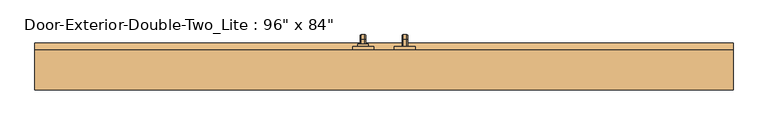
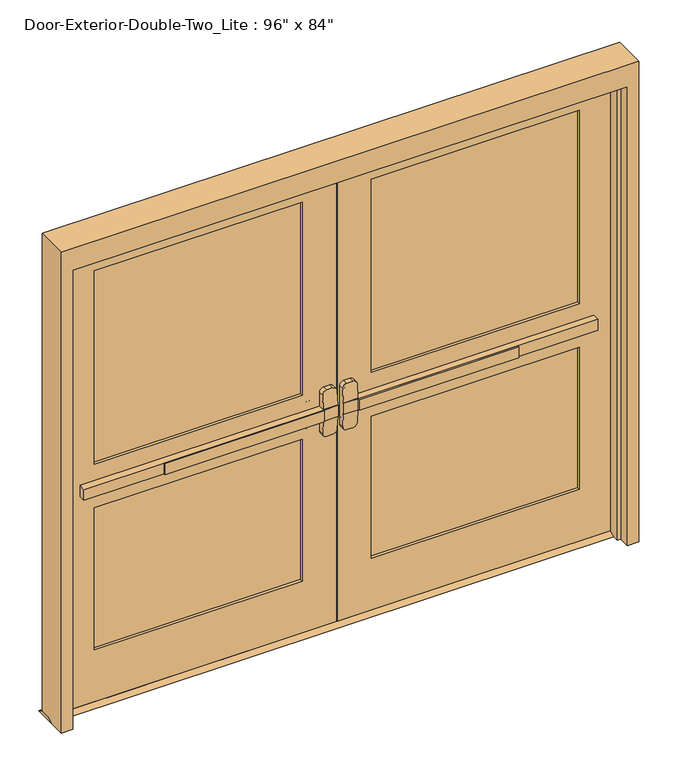
"""IFC4 building model written with IfcOpenShell, lengths in millimetres: door geometry."""

from ifc_helpers import new_model, si_unit, point, frame, frame_2d, origin, place, context, project, spatial, polyline, circle_curve, ellipse_curve, trimmed, segment, composite_curve, outline, extrude, faceted_brep, source, transform, mapped, element, save
from ifc_brep_helpers import plane_surface, cylinder_surface, revolved_surface, advanced_brep


def door_14451ac2(model_context):
    return source(origin(), model_context, "Body", "SolidModel", [
        extrude(outline(polyline([(-778.9333333, 0.0), (-778.9333333, 6.35), (-76.2, 6.35), (-76.2, 0.0), (-778.9333333, 0.0)])), frame((0.0, 0.0, 990.6), z_axis=(0.0, 0.0, 1.0), x_axis=(1.0, 0.0, 0.0)), (0.0, 0.0, 1.0), 50.8),
        advanced_brep(
        [(-12.7, 6.35, 1041.4), (-76.2, 6.35, 1041.4), (-1130.3, 6.35, 1041.4), (-1130.3, 6.35, 990.6), (-76.2, 6.35, 990.6), (-12.7, 6.35, 990.6), (-1130.3, 38.1, 1041.4), (-76.2, 38.1, 1041.4), (-76.2, 38.1, 1104.9), (-57.15, 38.1, 1123.95), (-31.75, 38.1, 1123.95), (-12.7, 38.1, 1104.9), (-12.7, 38.1, 927.1), (-31.75, 38.1, 908.05), (-57.15, 38.1, 908.05), (-76.2, 38.1, 927.1), (-76.2, 38.1, 990.6), (-1130.3, 38.1, 990.6), (-12.7, 9.5252467, 1041.4), (-76.2, 9.5252467, 1041.4), (-12.7, 9.5252467, 990.6), (-12.7, 14.5354269, 927.1), (-12.7, 14.5354269, 1104.9), (-76.2, 9.5252467, 990.6), (-76.2, 14.5354269, 1104.9), (-76.2, 14.5354269, 927.1), (-57.15, 16.038481, 1123.95), (-31.75, 16.038481, 1123.95), (-31.75, 16.038481, 908.05), (-57.15, 16.038481, 908.05)],
        [
            (0, 1),
            (1, 2),
            (2, 3),
            (3, 4),
            (4, 5),
            (5, 0),
            (6, 7),
            (7, 8),
            (8, 9, circle_curve(frame((-57.15, 38.1, 1104.9), z_axis=(0.0, 1.0, 0.0), x_axis=(-1.0, 0.0, 0.0)), 19.05)),
            (9, 10),
            (10, 11, circle_curve(frame((-31.75, 38.1, 1104.9), z_axis=(0.0, 1.0, 0.0), x_axis=(-1.0, 0.0, 0.0)), 19.05)),
            (11, 12),
            (12, 13, circle_curve(frame((-31.75, 38.1, 927.1), z_axis=(0.0, 1.0, 0.0), x_axis=(-1.0, 0.0, 0.0)), 19.05)),
            (13, 14),
            (14, 15, circle_curve(frame((-57.15, 38.1, 927.1), z_axis=(0.0, 1.0, 0.0), x_axis=(-1.0, 0.0, 0.0)), 19.05)),
            (15, 16),
            (16, 17),
            (17, 6),
            (0, 18),
            (18, 19),
            (19, 7),
            (6, 2),
            (5, 20),
            (20, 21),
            (21, 12),
            (11, 22),
            (22, 18),
            (16, 23),
            (23, 20),
            (3, 17),
            (19, 24),
            (24, 8),
            (15, 25),
            (25, 23),
            (9, 26),
            (26, 27),
            (27, 10),
            (13, 28),
            (28, 29),
            (29, 14),
            (29, 25, ellipse_curve(frame((-57.15, 14.5354269, 927.1), z_axis=(0.0, 0.9969018152893365, 0.07865602756830282), x_axis=(0.0, -0.07865602756830208, 0.9969018152893365)), 19.1092038, 19.05)),
            (24, 26, ellipse_curve(frame((-57.15, 14.5354269, 1104.9), z_axis=(0.0, 0.9969018152893376, -0.07865602756828934), x_axis=(0.0, -0.078656027568288, -0.9969018152893377)), 19.1092038, 19.05)),
            (27, 22, ellipse_curve(frame((-31.75, 14.5354269, 1104.9), z_axis=(0.0, 0.9969018152893376, -0.07865602756828934), x_axis=(0.0, -0.078656027568288, -0.9969018152893377)), 19.1092038, 19.05)),
            (21, 28, ellipse_curve(frame((-31.75, 14.5354269, 927.1), z_axis=(0.0, 0.9969018152893365, 0.07865602756830282), x_axis=(0.0, -0.07865602756830208, 0.9969018152893365)), 19.1092038, 19.05)),
        ],
        [
            plane_surface(frame((-12.7, 6.35, 1041.4), z_axis=(0.0, -1.0, 0.0), x_axis=(1.0, 0.0, 0.0))),
            plane_surface(frame((-12.7, 38.1, 1041.4), z_axis=(0.0, 1.0, 0.0), x_axis=(-1.0, 0.0, 0.0))),
            plane_surface(frame((-1130.3, 6.35, 1041.4), z_axis=(0.0, 0.0, 1.0), x_axis=(0.0, 1.0, 0.0))),
            plane_surface(frame((-12.7, 6.35, 1041.4), z_axis=(1.0, 0.0, 0.0), x_axis=(0.0, 1.0, 0.0))),
            plane_surface(frame((-12.7, 6.35, 990.6), z_axis=(0.0, 0.0, -1.0), x_axis=(0.0, 1.0, 0.0))),
            plane_surface(frame((-1130.3, 6.35, 990.6), z_axis=(-1.0, 0.0, 0.0), x_axis=(0.0, 1.0, 0.0))),
            plane_surface(frame((-76.2, 9.5252467, 927.1), z_axis=(-1.0, 0.0, 0.0), x_axis=(0.0, 1.0, 0.0))),
            plane_surface(frame((-57.15, 9.5252467, 1123.95), z_axis=(0.0, 0.0, 1.0), x_axis=(0.0, 1.0, 0.0))),
            plane_surface(frame((-31.75, 9.5252467, 908.05), z_axis=(0.0, 0.0, -1.0), x_axis=(0.0, 1.0, 0.0))),
            cylinder_surface(frame((-57.15, 38.1, 927.1), z_axis=(0.0, -1.0, 0.0), x_axis=(-1.0, 0.0, 0.0)), 19.05),
            cylinder_surface(frame((-57.15, 38.1, 1104.9), z_axis=(0.0, -1.0, 0.0), x_axis=(-1.0, 0.0, 0.0)), 19.05),
            cylinder_surface(frame((-31.75, 38.1, 1104.9), z_axis=(0.0, -1.0, 0.0), x_axis=(-1.0, 0.0, 0.0)), 19.05),
            cylinder_surface(frame((-31.75, 38.1, 927.1), z_axis=(0.0, -1.0, 0.0), x_axis=(-1.0, 0.0, 0.0)), 19.05),
            plane_surface(frame((-76.2, 9.5252467, 1041.4), z_axis=(0.0, -0.9969018152893376, 0.07865602756828934), x_axis=(1.0, 0.0, 0.0))),
            plane_surface(frame((-76.2, 16.038481, 908.05), z_axis=(0.0, -0.9969018152893365, -0.07865602756830282), x_axis=(1.0, 0.0, 0.0))),
        ],
        [
            (0, [[1, 2, 3, 4, 5, 6]]),
            (1, [[7, 8, 9, 10, 11, 12, 13, 14, 15, 16, 17, 18]]),
            (2, [[-2, -1, 19, 20, 21, -7, 22]]),
            (3, [[23, 24, 25, -12, 26, 27, -19, -6]]),
            (4, [[-17, 28, 29, -23, -5, -4, 30]]),
            (5, [[-22, -18, -30, -3]]),
            (6, [[-21, 31, 32, -8]]),
            (6, [[33, 34, -28, -16]]),
            (7, [[35, 36, 37, -10]]),
            (8, [[38, 39, 40, -14]]),
            (9, [[-40, 41, -33, -15]]),
            (10, [[-32, 42, -35, -9]]),
            (11, [[-37, 43, -26, -11]]),
            (12, [[-25, 44, -38, -13]]),
            (13, [[-27, -43, -36, -42, -31, -20]]),
            (14, [[-29, -34, -41, -39, -44, -24]]),
        ],
    ),
        extrude(outline(polyline([(82.55, 12.7), (107.95, 0.0), (12.7, 0.0), (38.1, 12.7), (82.55, 12.7)])), frame((-1270.0, 0.0, 0.0), z_axis=(1.0, 0.0, 0.0), x_axis=(0.0, 1.0, 0.0)), (0.0, 0.0, 1.0), 2540.0),
        extrude(outline(polyline([(778.9333333, 0.0), (76.2, 0.0), (76.2, 6.35), (778.9333333, 6.35), (778.9333333, 0.0)])), frame((0.0, 0.0, 990.6), z_axis=(0.0, 0.0, 1.0), x_axis=(1.0, 0.0, 0.0)), (0.0, 0.0, 1.0), 50.8),
        advanced_brep(
        [(12.7, 6.35, 1041.4), (12.7, 6.35, 990.6), (76.2, 6.35, 990.6), (1130.3, 6.35, 990.6), (1130.3, 6.35, 1041.4), (76.2, 6.35, 1041.4), (1130.3, 38.1, 1041.4), (1130.3, 38.1, 990.6), (76.2, 38.1, 990.6), (76.2, 38.1, 927.1), (57.15, 38.1, 908.05), (31.75, 38.1, 908.05), (12.7, 38.1, 927.1), (12.7, 38.1, 1104.9), (31.75, 38.1, 1123.95), (57.15, 38.1, 1123.95), (76.2, 38.1, 1104.9), (76.2, 38.1, 1041.4), (76.2, 9.5252467, 1041.4), (12.7, 9.5252467, 1041.4), (12.7, 14.5354269, 1104.9), (12.7, 14.5354269, 927.1), (12.7, 9.5252467, 990.6), (76.2, 9.5252467, 990.6), (76.2, 14.5354269, 927.1), (76.2, 14.5354269, 1104.9), (31.75, 16.038481, 1123.95), (57.15, 16.038481, 1123.95), (57.15, 16.038481, 908.05), (31.75, 16.038481, 908.05)],
        [
            (0, 1),
            (1, 2),
            (2, 3),
            (3, 4),
            (4, 5),
            (5, 0),
            (6, 7),
            (7, 8),
            (8, 9),
            (9, 10, circle_curve(frame((57.15, 38.1, 927.1), z_axis=(0.0, 1.0, 0.0), x_axis=(1.0, 0.0, 0.0)), 19.05)),
            (10, 11),
            (11, 12, circle_curve(frame((31.75, 38.1, 927.1), z_axis=(0.0, 1.0, 0.0), x_axis=(1.0, 0.0, 0.0)), 19.05)),
            (12, 13),
            (13, 14, circle_curve(frame((31.75, 38.1, 1104.9), z_axis=(0.0, 1.0, 0.0), x_axis=(1.0, 0.0, 0.0)), 19.05)),
            (14, 15),
            (15, 16, circle_curve(frame((57.15, 38.1, 1104.9), z_axis=(0.0, 1.0, 0.0), x_axis=(1.0, 0.0, 0.0)), 19.05)),
            (16, 17),
            (17, 6),
            (4, 6),
            (17, 18),
            (18, 19),
            (19, 0),
            (19, 20),
            (20, 13),
            (12, 21),
            (21, 22),
            (22, 1),
            (7, 3),
            (22, 23),
            (23, 8),
            (23, 24),
            (24, 9),
            (16, 25),
            (25, 18),
            (14, 26),
            (26, 27),
            (27, 15),
            (10, 28),
            (28, 29),
            (29, 11),
            (24, 28, ellipse_curve(frame((57.15, 14.5354269, 927.1), z_axis=(0.0, 0.9969018152893365, 0.07865602756830282), x_axis=(0.0, -0.07865602756830208, 0.9969018152893365)), 19.1092038, 19.05)),
            (27, 25, ellipse_curve(frame((57.15, 14.5354269, 1104.9), z_axis=(0.0, 0.9969018152893376, -0.07865602756828934), x_axis=(0.0, -0.078656027568288, -0.9969018152893377)), 19.1092038, 19.05)),
            (20, 26, ellipse_curve(frame((31.75, 14.5354269, 1104.9), z_axis=(0.0, 0.9969018152893376, -0.07865602756828934), x_axis=(0.0, -0.078656027568288, -0.9969018152893377)), 19.1092038, 19.05)),
            (29, 21, ellipse_curve(frame((31.75, 14.5354269, 927.1), z_axis=(0.0, 0.9969018152893365, 0.07865602756830282), x_axis=(0.0, -0.07865602756830208, 0.9969018152893365)), 19.1092038, 19.05)),
        ],
        [
            plane_surface(frame((12.7, 6.35, 1041.4), z_axis=(0.0, -1.0, 0.0), x_axis=(-1.0, 0.0, 0.0))),
            plane_surface(frame((12.7, 38.1, 1041.4), z_axis=(0.0, 1.0, 0.0), x_axis=(1.0, 0.0, 0.0))),
            plane_surface(frame((1130.3, 6.35, 1041.4), z_axis=(0.0, 0.0, 1.0), x_axis=(0.0, 1.0, 0.0))),
            plane_surface(frame((12.7, 6.35, 1041.4), z_axis=(-1.0, 0.0, 0.0), x_axis=(0.0, 1.0, 0.0))),
            plane_surface(frame((12.7, 6.35, 990.6), z_axis=(0.0, 0.0, -1.0), x_axis=(0.0, 1.0, 0.0))),
            plane_surface(frame((1130.3, 6.35, 990.6), z_axis=(1.0, 0.0, 0.0), x_axis=(0.0, 1.0, 0.0))),
            plane_surface(frame((76.2, 9.5252467, 927.1), z_axis=(1.0, 0.0, 0.0), x_axis=(0.0, 1.0, 0.0))),
            plane_surface(frame((57.15, 9.5252467, 1123.95), z_axis=(0.0, 0.0, 1.0), x_axis=(0.0, 1.0, 0.0))),
            plane_surface(frame((31.75, 9.5252467, 908.05), z_axis=(0.0, 0.0, -1.0), x_axis=(0.0, 1.0, 0.0))),
            cylinder_surface(frame((57.15, 38.1, 927.1), z_axis=(0.0, -1.0, 0.0), x_axis=(1.0, 0.0, 0.0)), 19.05),
            cylinder_surface(frame((57.15, 38.1, 1104.9), z_axis=(0.0, -1.0, 0.0), x_axis=(1.0, 0.0, 0.0)), 19.05),
            cylinder_surface(frame((31.75, 38.1, 1104.9), z_axis=(0.0, -1.0, 0.0), x_axis=(1.0, 0.0, 0.0)), 19.05),
            cylinder_surface(frame((31.75, 38.1, 927.1), z_axis=(0.0, -1.0, 0.0), x_axis=(1.0, 0.0, 0.0)), 19.05),
            plane_surface(frame((76.2, 9.5252467, 1041.4), z_axis=(0.0, -0.9969018152893376, 0.07865602756828934), x_axis=(-1.0, 0.0, 0.0))),
            plane_surface(frame((76.2, 16.038481, 908.05), z_axis=(0.0, -0.9969018152893365, -0.07865602756830282), x_axis=(-1.0, 0.0, 0.0))),
        ],
        [
            (0, [[1, 2, 3, 4, 5, 6]]),
            (1, [[7, 8, 9, 10, 11, 12, 13, 14, 15, 16, 17, 18]]),
            (2, [[19, -18, 20, 21, 22, -6, -5]]),
            (3, [[-1, -22, 23, 24, -13, 25, 26, 27]]),
            (4, [[28, -3, -2, -27, 29, 30, -8]]),
            (5, [[-4, -28, -7, -19]]),
            (6, [[-9, -30, 31, 32]]),
            (6, [[-17, 33, 34, -20]]),
            (7, [[-15, 35, 36, 37]]),
            (8, [[-11, 38, 39, 40]]),
            (9, [[-10, -32, 41, -38]]),
            (10, [[-16, -37, 42, -33]]),
            (11, [[-14, -24, 43, -35]]),
            (12, [[-12, -40, 44, -25]]),
            (13, [[-21, -34, -42, -36, -43, -23]]),
            (14, [[-26, -44, -39, -41, -31, -29]]),
        ],
    ),
        advanced_brep(
        [(66.2, 95.25, 1017.190625), (66.2, 95.25, 1014.809375), (69.771875, 95.25, 1011.2375), (82.6284594, 95.25, 1011.2375), (86.2, 95.25, 1014.8090406), (86.2, 95.25, 1017.190625), (82.628125, 95.25, 1020.7625), (69.771875, 95.25, 1020.7625), (66.2, 95.25, 887.809375), (69.771875, 95.25, 884.2375), (82.628125, 95.25, 884.2375), (86.2, 95.25, 887.809375), (86.2, 95.25, 890.1909594), (82.6284594, 95.25, 893.7625), (69.771875, 95.25, 893.7625), (66.2, 95.25, 890.190625), (66.2, 120.65, 1017.190625), (66.2, 134.540625, 1003.3), (66.2, 134.540625, 901.7), (66.2, 120.65, 887.809375), (66.2, 120.65, 890.190625), (66.2, 132.159375, 901.7), (66.2, 132.159375, 1003.3), (66.2, 120.65, 1014.809375), (69.771875, 120.65, 1011.2375), (82.6284594, 120.65, 1011.2375), (86.2, 120.65, 1014.8090406), (86.2, 132.1590406, 1003.3), (86.2, 132.1590406, 901.7), (86.2, 120.65, 890.1909594), (86.2, 120.65, 887.809375), (86.2, 134.540625, 901.7), (86.2, 134.540625, 1003.3), (86.2, 120.65, 1017.190625), (82.628125, 120.65, 1020.7625), (69.771875, 120.65, 1020.7625), (69.771875, 128.5875, 1003.3), (82.6284594, 128.5875, 1003.3), (82.628125, 138.1125, 1003.3), (69.771875, 138.1125, 1003.3), (69.771875, 128.5875, 901.7), (82.6284594, 128.5875, 901.7), (82.628125, 138.1125, 901.7), (69.771875, 138.1125, 901.7), (69.771875, 120.65, 893.7625), (82.6284594, 120.65, 893.7625), (82.628125, 120.65, 884.2375), (69.771875, 120.65, 884.2375)],
        [
            (0, 1),
            (1, 2, circle_curve(frame((69.771875, 95.25, 1014.809375), z_axis=(0.0, -1.0, 0.0), x_axis=(0.0, 0.0, 1.0)), 3.571875)),
            (2, 3),
            (3, 4, circle_curve(frame((82.6284594, 95.25, 1014.8090406), z_axis=(0.0, -1.0, 0.0), x_axis=(0.0, 0.0, 1.0)), 3.5715406)),
            (4, 5),
            (5, 6, circle_curve(frame((82.628125, 95.25, 1017.190625), z_axis=(0.0, -1.0, 0.0), x_axis=(0.0, 0.0, 1.0)), 3.571875)),
            (6, 7),
            (7, 0, circle_curve(frame((69.771875, 95.25, 1017.190625), z_axis=(0.0, -1.0, 0.0), x_axis=(0.0, 0.0, 1.0)), 3.571875)),
            (8, 9, circle_curve(frame((69.771875, 95.25, 887.809375), z_axis=(0.0, -1.0, 0.0), x_axis=(0.0, 0.0, -1.0)), 3.571875)),
            (9, 10),
            (10, 11, circle_curve(frame((82.628125, 95.25, 887.809375), z_axis=(0.0, -1.0, 0.0), x_axis=(0.0, 0.0, -1.0)), 3.571875)),
            (11, 12),
            (12, 13, circle_curve(frame((82.6284594, 95.25, 890.1909594), z_axis=(0.0, -1.0, 0.0), x_axis=(0.0, 0.0, -1.0)), 3.5715406)),
            (13, 14),
            (14, 15, circle_curve(frame((69.771875, 95.25, 890.190625), z_axis=(0.0, -1.0, 0.0), x_axis=(0.0, 0.0, -1.0)), 3.571875)),
            (15, 8),
            (0, 16),
            (16, 17, circle_curve(frame((66.2, 120.65, 1003.3), z_axis=(-1.0, 0.0, 0.0), x_axis=(0.0, 0.0, 1.0)), 13.890625)),
            (17, 18),
            (18, 19, circle_curve(frame((66.2, 120.65, 901.7), z_axis=(-1.0, 0.0, 0.0), x_axis=(0.0, 1.0, 0.0)), 13.890625)),
            (19, 8),
            (15, 20),
            (20, 21, circle_curve(frame((66.2, 120.65, 901.7), z_axis=(1.0, 0.0, 0.0), x_axis=(0.0, 1.0, 0.0)), 11.509375)),
            (21, 22),
            (22, 23, circle_curve(frame((66.2, 120.65, 1003.3), z_axis=(1.0, 0.0, 0.0), x_axis=(0.0, 0.0, 1.0)), 11.509375)),
            (23, 1),
            (23, 24, circle_curve(frame((69.771875, 120.65, 1014.809375), z_axis=(0.0, -1.0, 0.0), x_axis=(0.0, 0.0, 1.0)), 3.571875)),
            (24, 2),
            (24, 25),
            (25, 3),
            (25, 26, circle_curve(frame((82.6284594, 120.65, 1014.8090406), z_axis=(0.0, -1.0, 0.0), x_axis=(0.0, 0.0, 1.0)), 3.5715406)),
            (26, 4),
            (26, 27, circle_curve(frame((86.2, 120.65, 1003.3), z_axis=(-1.0, 0.0, 0.0), x_axis=(0.0, 0.0, 1.0)), 11.5090406)),
            (27, 28),
            (28, 29, circle_curve(frame((86.2, 120.65, 901.7), z_axis=(-1.0, 0.0, 0.0), x_axis=(0.0, 1.0, 0.0)), 11.5090406)),
            (29, 12),
            (11, 30),
            (30, 31, circle_curve(frame((86.2, 120.65, 901.7), z_axis=(1.0, 0.0, 0.0), x_axis=(0.0, 1.0, 0.0)), 13.890625)),
            (31, 32),
            (32, 33, circle_curve(frame((86.2, 120.65, 1003.3), z_axis=(1.0, 0.0, 0.0), x_axis=(0.0, 0.0, 1.0)), 13.890625)),
            (33, 5),
            (33, 34, circle_curve(frame((82.628125, 120.65, 1017.190625), z_axis=(0.0, -1.0, 0.0), x_axis=(0.0, 0.0, 1.0)), 3.571875)),
            (34, 6),
            (34, 35),
            (35, 7),
            (35, 16, circle_curve(frame((69.771875, 120.65, 1017.190625), z_axis=(0.0, -1.0, 0.0), x_axis=(0.0, 0.0, 1.0)), 3.571875)),
            (36, 24, circle_curve(frame((69.771875, 120.65, 1003.3), z_axis=(1.0, 0.0, 0.0), x_axis=(0.0, 0.0, 1.0)), 7.9375)),
            (22, 36, circle_curve(frame((69.771875, 132.159375, 1003.3), z_axis=(0.0, 0.0, 1.0), x_axis=(0.0, 1.0, 0.0)), 3.571875)),
            (37, 25, circle_curve(frame((82.6284594, 120.65, 1003.3), z_axis=(1.0, 0.0, 0.0), x_axis=(0.0, 0.0, 1.0)), 7.9375)),
            (36, 37),
            (37, 27, circle_curve(frame((82.6284594, 132.1590406, 1003.3), z_axis=(0.0, 0.0, 1.0), x_axis=(0.0, 1.0, 0.0)), 3.5715406)),
            (38, 34, circle_curve(frame((82.628125, 120.65, 1003.3), z_axis=(1.0, 0.0, 0.0), x_axis=(0.0, 0.0, 1.0)), 17.4625)),
            (32, 38, circle_curve(frame((82.628125, 134.540625, 1003.3), z_axis=(0.0, 0.0, 1.0), x_axis=(0.0, 1.0, 0.0)), 3.571875)),
            (39, 35, circle_curve(frame((69.771875, 120.65, 1003.3), z_axis=(1.0, 0.0, 0.0), x_axis=(0.0, 0.0, 1.0)), 17.4625)),
            (38, 39),
            (39, 17, circle_curve(frame((69.771875, 134.540625, 1003.3), z_axis=(0.0, 0.0, 1.0), x_axis=(0.0, 1.0, 0.0)), 3.571875)),
            (21, 40, circle_curve(frame((69.771875, 132.159375, 901.7), z_axis=(0.0, 0.0, 1.0), x_axis=(0.0, 1.0, 0.0)), 3.571875)),
            (40, 36),
            (40, 41),
            (41, 37),
            (41, 28, circle_curve(frame((82.6284594, 132.1590406, 901.7), z_axis=(0.0, 0.0, 1.0), x_axis=(0.0, 1.0, 0.0)), 3.5715406)),
            (31, 42, circle_curve(frame((82.628125, 134.540625, 901.7), z_axis=(0.0, 0.0, 1.0), x_axis=(0.0, 1.0, 0.0)), 3.571875)),
            (42, 38),
            (42, 43),
            (43, 39),
            (43, 18, circle_curve(frame((69.771875, 134.540625, 901.7), z_axis=(0.0, 0.0, 1.0), x_axis=(0.0, 1.0, 0.0)), 3.571875)),
            (44, 40, circle_curve(frame((69.771875, 120.65, 901.7), z_axis=(1.0, 0.0, 0.0), x_axis=(0.0, 1.0, 0.0)), 7.9375)),
            (20, 44, circle_curve(frame((69.771875, 120.65, 890.190625), z_axis=(0.0, 1.0, 0.0), x_axis=(0.0, 0.0, -1.0)), 3.571875)),
            (45, 41, circle_curve(frame((82.6284594, 120.65, 901.7), z_axis=(1.0, 0.0, 0.0), x_axis=(0.0, 1.0, 0.0)), 7.9375)),
            (44, 45),
            (45, 29, circle_curve(frame((82.6284594, 120.65, 890.1909594), z_axis=(0.0, 1.0, 0.0), x_axis=(0.0, 0.0, -1.0)), 3.5715406)),
            (46, 42, circle_curve(frame((82.628125, 120.65, 901.7), z_axis=(1.0, 0.0, 0.0), x_axis=(0.0, 1.0, 0.0)), 17.4625)),
            (30, 46, circle_curve(frame((82.628125, 120.65, 887.809375), z_axis=(0.0, 1.0, 0.0), x_axis=(0.0, 0.0, -1.0)), 3.571875)),
            (47, 43, circle_curve(frame((69.771875, 120.65, 901.7), z_axis=(1.0, 0.0, 0.0), x_axis=(0.0, 1.0, 0.0)), 17.4625)),
            (46, 47),
            (47, 19, circle_curve(frame((69.771875, 120.65, 887.809375), z_axis=(0.0, 1.0, 0.0), x_axis=(0.0, 0.0, -1.0)), 3.571875)),
            (14, 44),
            (13, 45),
            (10, 46),
            (9, 47),
        ],
        [
            plane_surface(frame((76.2, 95.25, 1016.0), z_axis=(0.0, -1.0, 0.0), x_axis=(1.0, 0.0, 0.0))),
            plane_surface(frame((76.2, 95.25, 889.0), z_axis=(0.0, -1.0, 0.0), x_axis=(1.0, 0.0, 0.0))),
            plane_surface(frame((66.2, 95.25, 1017.190625), z_axis=(-1.0, 0.0, 0.0), x_axis=(0.0, 1.0, 0.0))),
            cylinder_surface(frame((69.771875, 95.25, 1014.809375), z_axis=(0.0, -1.0, 0.0), x_axis=(0.0, 0.0, 1.0)), 3.571875),
            plane_surface(frame((69.771875, 95.25, 1011.2375), z_axis=(0.0, 0.0, -1.0), x_axis=(0.0, 1.0, 0.0))),
            cylinder_surface(frame((82.6284594, 95.25, 1014.8090406), z_axis=(0.0, -1.0, 0.0), x_axis=(0.0, 0.0, 1.0)), 3.5715406),
            plane_surface(frame((86.2, 95.25, 1014.8090406), z_axis=(1.0, 0.0, 0.0), x_axis=(0.0, 1.0, 0.0))),
            cylinder_surface(frame((82.628125, 95.25, 1017.190625), z_axis=(0.0, -1.0, 0.0), x_axis=(0.0, 0.0, 1.0)), 3.571875),
            plane_surface(frame((82.628125, 95.25, 1020.7625), z_axis=(0.0, 0.0, 1.0), x_axis=(0.0, 1.0, 0.0))),
            cylinder_surface(frame((69.771875, 95.25, 1017.190625), z_axis=(0.0, -1.0, 0.0), x_axis=(0.0, 0.0, 1.0)), 3.571875),
            revolved_surface(trimmed(ellipse_curve(frame((69.771875, 120.65, 1014.809375), z_axis=(0.0, -1.0, 0.0), x_axis=(0.0, 0.0, 1.0)), 3.571875, 3.571875), [point((66.2, 120.65, 1014.809375))], [point((69.771875, 120.65, 1011.2375))], True, "CARTESIAN"), (76.2, 120.65, 1003.3), (-1.0, 0.0, 0.0)),
            revolved_surface(polyline([(69.771875, 120.65, 1011.2375), (82.6284594, 120.65, 1011.2375)]), (76.2, 120.65, 1003.3), (-1.0, 0.0, 0.0)),
            revolved_surface(trimmed(ellipse_curve(frame((82.6284594, 120.65, 1014.8090406), z_axis=(0.0, -1.0, 0.0), x_axis=(0.0, 0.0, 1.0)), 3.5715406, 3.5715406), [point((82.6284594, 120.65, 1011.2375))], [point((86.2, 120.65, 1014.8090406))], True, "CARTESIAN"), (76.2, 120.65, 1003.3), (-1.0, 0.0, 0.0)),
            revolved_surface(trimmed(ellipse_curve(frame((82.628125, 120.65, 1017.190625), z_axis=(0.0, -1.0, 0.0), x_axis=(0.0, 0.0, 1.0)), 3.571875, 3.571875), [point((86.2, 120.65, 1017.190625))], [point((82.628125, 120.65, 1020.7625))], True, "CARTESIAN"), (76.2, 120.65, 1003.3), (-1.0, 0.0, 0.0)),
            cylinder_surface(frame((76.2, 120.65, 1003.3), z_axis=(-1.0, 0.0, 0.0), x_axis=(0.0, 0.0, 1.0)), 17.4625),
            revolved_surface(trimmed(ellipse_curve(frame((69.771875, 120.65, 1017.190625), z_axis=(0.0, -1.0, 0.0), x_axis=(0.0, 0.0, 1.0)), 3.571875, 3.571875), [point((69.771875, 120.65, 1020.7625))], [point((66.2, 120.65, 1017.190625))], True, "CARTESIAN"), (76.2, 120.65, 1003.3), (-1.0, 0.0, 0.0)),
            cylinder_surface(frame((69.771875, 132.159375, 1003.3), z_axis=(0.0, 0.0, 1.0), x_axis=(0.0, 1.0, 0.0)), 3.571875),
            plane_surface(frame((69.771875, 128.5875, 1003.3), z_axis=(0.0, -1.0, 0.0), x_axis=(0.0, 0.0, -1.0))),
            cylinder_surface(frame((82.6284594, 132.1590406, 1003.3), z_axis=(0.0, 0.0, 1.0), x_axis=(0.0, 1.0, 0.0)), 3.5715406),
            cylinder_surface(frame((82.628125, 134.540625, 1003.3), z_axis=(0.0, 0.0, 1.0), x_axis=(0.0, 1.0, 0.0)), 3.571875),
            plane_surface(frame((82.628125, 138.1125, 1003.3), z_axis=(0.0, 1.0, 0.0), x_axis=(0.0, 0.0, -1.0))),
            cylinder_surface(frame((69.771875, 134.540625, 1003.3), z_axis=(0.0, 0.0, 1.0), x_axis=(0.0, 1.0, 0.0)), 3.571875),
            revolved_surface(trimmed(ellipse_curve(frame((69.771875, 132.159375, 901.7), z_axis=(0.0, 0.0, 1.0), x_axis=(0.0, 1.0, 0.0)), 3.571875, 3.571875), [point((66.2, 132.159375, 901.7))], [point((69.771875, 128.5875, 901.7))], True, "CARTESIAN"), (76.2, 120.65, 901.7), (-1.0, 0.0, 0.0)),
            revolved_surface(polyline([(69.771875, 128.5875, 901.7), (82.6284594, 128.5875, 901.7)]), (76.2, 120.65, 901.7), (-1.0, 0.0, 0.0)),
            revolved_surface(trimmed(ellipse_curve(frame((82.6284594, 132.1590406, 901.7), z_axis=(0.0, 0.0, 1.0), x_axis=(0.0, 1.0, 0.0)), 3.5715406, 3.5715406), [point((82.6284594, 128.5875, 901.7))], [point((86.2, 132.1590406, 901.7))], True, "CARTESIAN"), (76.2, 120.65, 901.7), (-1.0, 0.0, 0.0)),
            revolved_surface(trimmed(ellipse_curve(frame((82.628125, 134.540625, 901.7), z_axis=(0.0, 0.0, 1.0), x_axis=(0.0, 1.0, 0.0)), 3.571875, 3.571875), [point((86.2, 134.540625, 901.7))], [point((82.628125, 138.1125, 901.7))], True, "CARTESIAN"), (76.2, 120.65, 901.7), (-1.0, 0.0, 0.0)),
            cylinder_surface(frame((76.2, 120.65, 901.7), z_axis=(-1.0, 0.0, 0.0), x_axis=(0.0, 1.0, 0.0)), 17.4625),
            revolved_surface(trimmed(ellipse_curve(frame((69.771875, 134.540625, 901.7), z_axis=(0.0, 0.0, 1.0), x_axis=(0.0, 1.0, 0.0)), 3.571875, 3.571875), [point((69.771875, 138.1125, 901.7))], [point((66.2, 134.540625, 901.7))], True, "CARTESIAN"), (76.2, 120.65, 901.7), (-1.0, 0.0, 0.0)),
            cylinder_surface(frame((69.771875, 120.65, 890.190625), z_axis=(0.0, 1.0, 0.0), x_axis=(0.0, 0.0, -1.0)), 3.571875),
            plane_surface(frame((69.771875, 120.65, 893.7625), z_axis=(0.0, 0.0, 1.0), x_axis=(0.0, -1.0, 0.0))),
            cylinder_surface(frame((82.6284594, 120.65, 890.1909594), z_axis=(0.0, 1.0, 0.0), x_axis=(0.0, 0.0, -1.0)), 3.5715406),
            cylinder_surface(frame((82.628125, 120.65, 887.809375), z_axis=(0.0, 1.0, 0.0), x_axis=(0.0, 0.0, -1.0)), 3.571875),
            plane_surface(frame((82.628125, 120.65, 884.2375), z_axis=(0.0, 0.0, -1.0), x_axis=(0.0, -1.0, 0.0))),
            cylinder_surface(frame((69.771875, 120.65, 887.809375), z_axis=(0.0, 1.0, 0.0), x_axis=(0.0, 0.0, -1.0)), 3.571875),
        ],
        [
            (0, [[1, 2, 3, 4, 5, 6, 7, 8]]),
            (1, [[9, 10, 11, 12, 13, 14, 15, 16]]),
            (2, [[-1, 17, 18, 19, 20, 21, -16, 22, 23, 24, 25, 26]]),
            (3, [[-2, -26, 27, 28]]),
            (4, [[-3, -28, 29, 30]]),
            (5, [[-4, -30, 31, 32]]),
            (6, [[-5, -32, 33, 34, 35, 36, -12, 37, 38, 39, 40, 41]]),
            (7, [[-6, -41, 42, 43]]),
            (8, [[-7, -43, 44, 45]]),
            (9, [[-8, -45, 46, -17]]),
            (10, [[47, -27, -25, 48]]),
            (11, [[49, -29, -47, 50]]),
            (12, [[-33, -31, -49, 51]]),
            (13, [[52, -42, -40, 53]]),
            (14, [[54, -44, -52, 55]]),
            (15, [[-18, -46, -54, 56]]),
            (16, [[-48, -24, 57, 58]]),
            (17, [[-50, -58, 59, 60]]),
            (18, [[-51, -60, 61, -34]]),
            (19, [[-53, -39, 62, 63]]),
            (20, [[-55, -63, 64, 65]]),
            (21, [[-56, -65, 66, -19]]),
            (22, [[67, -57, -23, 68]]),
            (23, [[69, -59, -67, 70]]),
            (24, [[-35, -61, -69, 71]]),
            (25, [[72, -62, -38, 73]]),
            (26, [[74, -64, -72, 75]]),
            (27, [[-20, -66, -74, 76]]),
            (28, [[-68, -22, -15, 77]]),
            (29, [[-70, -77, -14, 78]]),
            (30, [[-71, -78, -13, -36]]),
            (31, [[-73, -37, -11, 79]]),
            (32, [[-75, -79, -10, 80]]),
            (33, [[-76, -80, -9, -21]]),
        ],
    ),
        extrude(outline(composite_curve([segment(trimmed(circle_curve(frame_2d((1113.0338574, 76.2)), 89.3016225), [point((1193.8, 114.3))], [point((1193.8, 38.1))], False, "CARTESIAN"), True, "CONTINUOUS"), segment(polyline([(1193.8, 38.1), (838.2, 38.1)]), True, "CONTINUOUS"), segment(trimmed(circle_curve(frame_2d((918.9661426, 76.2)), 89.3016225), [point((838.2, 38.1))], [point((838.2, 114.3))], False, "CARTESIAN"), True, "CONTINUOUS"), segment(polyline([(838.2, 114.3), (1193.8, 114.3)]), True, "CONTINUOUS")], self_intersect=False)), frame((0.0, 82.55, 0.0), z_axis=(0.0, 1.0, 0.0), x_axis=(0.0, 0.0, 1.0)), (0.0, 0.0, 1.0), 12.7),
        advanced_brep(
        [(-86.2, 95.25, 1017.190625), (-86.2, 95.25, 1014.809375), (-82.628125, 95.25, 1011.2375), (-69.7715406, 95.25, 1011.2375), (-66.2, 95.25, 1014.8090406), (-66.2, 95.25, 1017.190625), (-69.771875, 95.25, 1020.7625), (-82.628125, 95.25, 1020.7625), (-86.2, 95.25, 887.809375), (-82.628125, 95.25, 884.2375), (-69.771875, 95.25, 884.2375), (-66.2, 95.25, 887.809375), (-66.2, 95.25, 890.1909594), (-69.7715406, 95.25, 893.7625), (-82.628125, 95.25, 893.7625), (-86.2, 95.25, 890.190625), (-86.2, 120.65, 1017.190625), (-86.2, 134.540625, 1003.3), (-86.2, 134.540625, 901.7), (-86.2, 120.65, 887.809375), (-86.2, 120.65, 890.190625), (-86.2, 132.159375, 901.7), (-86.2, 132.159375, 1003.3), (-86.2, 120.65, 1014.809375), (-82.628125, 120.65, 1011.2375), (-69.7715406, 120.65, 1011.2375), (-66.2, 120.65, 1014.8090406), (-66.2, 132.1590406, 1003.3), (-66.2, 132.1590406, 901.7), (-66.2, 120.65, 890.1909594), (-66.2, 120.65, 887.809375), (-66.2, 134.540625, 901.7), (-66.2, 134.540625, 1003.3), (-66.2, 120.65, 1017.190625), (-69.771875, 120.65, 1020.7625), (-82.628125, 120.65, 1020.7625), (-82.628125, 128.5875, 1003.3), (-69.7715406, 128.5875, 1003.3), (-69.771875, 138.1125, 1003.3), (-82.628125, 138.1125, 1003.3), (-82.628125, 128.5875, 901.7), (-69.7715406, 128.5875, 901.7), (-69.771875, 138.1125, 901.7), (-82.628125, 138.1125, 901.7), (-82.628125, 120.65, 893.7625), (-69.7715406, 120.65, 893.7625), (-69.771875, 120.65, 884.2375), (-82.628125, 120.65, 884.2375)],
        [
            (0, 1),
            (1, 2, circle_curve(frame((-82.628125, 95.25, 1014.809375), z_axis=(0.0, -1.0, 0.0), x_axis=(0.0, 0.0, 1.0)), 3.571875)),
            (2, 3),
            (3, 4, circle_curve(frame((-69.7715406, 95.25, 1014.8090406), z_axis=(0.0, -1.0, 0.0), x_axis=(0.0, 0.0, 1.0)), 3.5715406)),
            (4, 5),
            (5, 6, circle_curve(frame((-69.771875, 95.25, 1017.190625), z_axis=(0.0, -1.0, 0.0), x_axis=(0.0, 0.0, 1.0)), 3.571875)),
            (6, 7),
            (7, 0, circle_curve(frame((-82.628125, 95.25, 1017.190625), z_axis=(0.0, -1.0, 0.0), x_axis=(0.0, 0.0, 1.0)), 3.571875)),
            (8, 9, circle_curve(frame((-82.628125, 95.25, 887.809375), z_axis=(0.0, -1.0, 0.0), x_axis=(0.0, 0.0, -1.0)), 3.571875)),
            (9, 10),
            (10, 11, circle_curve(frame((-69.771875, 95.25, 887.809375), z_axis=(0.0, -1.0, 0.0), x_axis=(0.0, 0.0, -1.0)), 3.571875)),
            (11, 12),
            (12, 13, circle_curve(frame((-69.7715406, 95.25, 890.1909594), z_axis=(0.0, -1.0, 0.0), x_axis=(0.0, 0.0, -1.0)), 3.5715406)),
            (13, 14),
            (14, 15, circle_curve(frame((-82.628125, 95.25, 890.190625), z_axis=(0.0, -1.0, 0.0), x_axis=(0.0, 0.0, -1.0)), 3.571875)),
            (15, 8),
            (0, 16),
            (16, 17, circle_curve(frame((-86.2, 120.65, 1003.3), z_axis=(-1.0, 0.0, 0.0), x_axis=(0.0, 0.0, 1.0)), 13.890625)),
            (17, 18),
            (18, 19, circle_curve(frame((-86.2, 120.65, 901.7), z_axis=(-1.0, 0.0, 0.0), x_axis=(0.0, 1.0, 0.0)), 13.890625)),
            (19, 8),
            (15, 20),
            (20, 21, circle_curve(frame((-86.2, 120.65, 901.7), z_axis=(1.0, 0.0, 0.0), x_axis=(0.0, 1.0, 0.0)), 11.509375)),
            (21, 22),
            (22, 23, circle_curve(frame((-86.2, 120.65, 1003.3), z_axis=(1.0, 0.0, 0.0), x_axis=(0.0, 0.0, 1.0)), 11.509375)),
            (23, 1),
            (23, 24, circle_curve(frame((-82.628125, 120.65, 1014.809375), z_axis=(0.0, -1.0, 0.0), x_axis=(0.0, 0.0, 1.0)), 3.571875)),
            (24, 2),
            (24, 25),
            (25, 3),
            (25, 26, circle_curve(frame((-69.7715406, 120.65, 1014.8090406), z_axis=(0.0, -1.0, 0.0), x_axis=(0.0, 0.0, 1.0)), 3.5715406)),
            (26, 4),
            (26, 27, circle_curve(frame((-66.2, 120.65, 1003.3), z_axis=(-1.0, 0.0, 0.0), x_axis=(0.0, 0.0, 1.0)), 11.5090406)),
            (27, 28),
            (28, 29, circle_curve(frame((-66.2, 120.65, 901.7), z_axis=(-1.0, 0.0, 0.0), x_axis=(0.0, 1.0, 0.0)), 11.5090406)),
            (29, 12),
            (11, 30),
            (30, 31, circle_curve(frame((-66.2, 120.65, 901.7), z_axis=(1.0, 0.0, 0.0), x_axis=(0.0, 1.0, 0.0)), 13.890625)),
            (31, 32),
            (32, 33, circle_curve(frame((-66.2, 120.65, 1003.3), z_axis=(1.0, 0.0, 0.0), x_axis=(0.0, 0.0, 1.0)), 13.890625)),
            (33, 5),
            (33, 34, circle_curve(frame((-69.771875, 120.65, 1017.190625), z_axis=(0.0, -1.0, 0.0), x_axis=(0.0, 0.0, 1.0)), 3.571875)),
            (34, 6),
            (34, 35),
            (35, 7),
            (35, 16, circle_curve(frame((-82.628125, 120.65, 1017.190625), z_axis=(0.0, -1.0, 0.0), x_axis=(0.0, 0.0, 1.0)), 3.571875)),
            (36, 24, circle_curve(frame((-82.628125, 120.65, 1003.3), z_axis=(1.0, 0.0, 0.0), x_axis=(0.0, 0.0, 1.0)), 7.9375)),
            (22, 36, circle_curve(frame((-82.628125, 132.159375, 1003.3), z_axis=(0.0, 0.0, 1.0), x_axis=(0.0, 1.0, 0.0)), 3.571875)),
            (37, 25, circle_curve(frame((-69.7715406, 120.65, 1003.3), z_axis=(1.0, 0.0, 0.0), x_axis=(0.0, 0.0, 1.0)), 7.9375)),
            (36, 37),
            (37, 27, circle_curve(frame((-69.7715406, 132.1590406, 1003.3), z_axis=(0.0, 0.0, 1.0), x_axis=(0.0, 1.0, 0.0)), 3.5715406)),
            (38, 34, circle_curve(frame((-69.771875, 120.65, 1003.3), z_axis=(1.0, 0.0, 0.0), x_axis=(0.0, 0.0, 1.0)), 17.4625)),
            (32, 38, circle_curve(frame((-69.771875, 134.540625, 1003.3), z_axis=(0.0, 0.0, 1.0), x_axis=(0.0, 1.0, 0.0)), 3.571875)),
            (39, 35, circle_curve(frame((-82.628125, 120.65, 1003.3), z_axis=(1.0, 0.0, 0.0), x_axis=(0.0, 0.0, 1.0)), 17.4625)),
            (38, 39),
            (39, 17, circle_curve(frame((-82.628125, 134.540625, 1003.3), z_axis=(0.0, 0.0, 1.0), x_axis=(0.0, 1.0, 0.0)), 3.571875)),
            (21, 40, circle_curve(frame((-82.628125, 132.159375, 901.7), z_axis=(0.0, 0.0, 1.0), x_axis=(0.0, 1.0, 0.0)), 3.571875)),
            (40, 36),
            (40, 41),
            (41, 37),
            (41, 28, circle_curve(frame((-69.7715406, 132.1590406, 901.7), z_axis=(0.0, 0.0, 1.0), x_axis=(0.0, 1.0, 0.0)), 3.5715406)),
            (31, 42, circle_curve(frame((-69.771875, 134.540625, 901.7), z_axis=(0.0, 0.0, 1.0), x_axis=(0.0, 1.0, 0.0)), 3.571875)),
            (42, 38),
            (42, 43),
            (43, 39),
            (43, 18, circle_curve(frame((-82.628125, 134.540625, 901.7), z_axis=(0.0, 0.0, 1.0), x_axis=(0.0, 1.0, 0.0)), 3.571875)),
            (44, 40, circle_curve(frame((-82.628125, 120.65, 901.7), z_axis=(1.0, 0.0, 0.0), x_axis=(0.0, 1.0, 0.0)), 7.9375)),
            (20, 44, circle_curve(frame((-82.628125, 120.65, 890.190625), z_axis=(0.0, 1.0, 0.0), x_axis=(0.0, 0.0, -1.0)), 3.571875)),
            (45, 41, circle_curve(frame((-69.7715406, 120.65, 901.7), z_axis=(1.0, 0.0, 0.0), x_axis=(0.0, 1.0, 0.0)), 7.9375)),
            (44, 45),
            (45, 29, circle_curve(frame((-69.7715406, 120.65, 890.1909594), z_axis=(0.0, 1.0, 0.0), x_axis=(0.0, 0.0, -1.0)), 3.5715406)),
            (46, 42, circle_curve(frame((-69.771875, 120.65, 901.7), z_axis=(1.0, 0.0, 0.0), x_axis=(0.0, 1.0, 0.0)), 17.4625)),
            (30, 46, circle_curve(frame((-69.771875, 120.65, 887.809375), z_axis=(0.0, 1.0, 0.0), x_axis=(0.0, 0.0, -1.0)), 3.571875)),
            (47, 43, circle_curve(frame((-82.628125, 120.65, 901.7), z_axis=(1.0, 0.0, 0.0), x_axis=(0.0, 1.0, 0.0)), 17.4625)),
            (46, 47),
            (47, 19, circle_curve(frame((-82.628125, 120.65, 887.809375), z_axis=(0.0, 1.0, 0.0), x_axis=(0.0, 0.0, -1.0)), 3.571875)),
            (14, 44),
            (13, 45),
            (10, 46),
            (9, 47),
        ],
        [
            plane_surface(frame((-76.2, 95.25, 1016.0), z_axis=(0.0, -1.0, 0.0), x_axis=(1.0, 0.0, 0.0))),
            plane_surface(frame((-76.2, 95.25, 889.0), z_axis=(0.0, -1.0, 0.0), x_axis=(1.0, 0.0, 0.0))),
            plane_surface(frame((-86.2, 95.25, 1017.190625), z_axis=(-1.0, 0.0, 0.0), x_axis=(0.0, 1.0, 0.0))),
            cylinder_surface(frame((-82.628125, 95.25, 1014.809375), z_axis=(0.0, -1.0, 0.0), x_axis=(0.0, 0.0, 1.0)), 3.571875),
            plane_surface(frame((-82.628125, 95.25, 1011.2375), z_axis=(0.0, 0.0, -1.0), x_axis=(0.0, 1.0, 0.0))),
            cylinder_surface(frame((-69.7715406, 95.25, 1014.8090406), z_axis=(0.0, -1.0, 0.0), x_axis=(0.0, 0.0, 1.0)), 3.5715406),
            plane_surface(frame((-66.2, 95.25, 1014.8090406), z_axis=(1.0, 0.0, 0.0), x_axis=(0.0, 1.0, 0.0))),
            cylinder_surface(frame((-69.771875, 95.25, 1017.190625), z_axis=(0.0, -1.0, 0.0), x_axis=(0.0, 0.0, 1.0)), 3.571875),
            plane_surface(frame((-69.771875, 95.25, 1020.7625), z_axis=(0.0, 0.0, 1.0), x_axis=(0.0, 1.0, 0.0))),
            cylinder_surface(frame((-82.628125, 95.25, 1017.190625), z_axis=(0.0, -1.0, 0.0), x_axis=(0.0, 0.0, 1.0)), 3.571875),
            revolved_surface(trimmed(ellipse_curve(frame((-82.628125, 120.65, 1014.809375), z_axis=(0.0, -1.0, 0.0), x_axis=(0.0, 0.0, 1.0)), 3.571875, 3.571875), [point((-86.2, 120.65, 1014.809375))], [point((-82.628125, 120.65, 1011.2375))], True, "CARTESIAN"), (-76.2, 120.65, 1003.3), (-1.0, 0.0, 0.0)),
            revolved_surface(polyline([(-82.628125, 120.65, 1011.2375), (-69.7715406, 120.65, 1011.2375)]), (-76.2, 120.65, 1003.3), (-1.0, 0.0, 0.0)),
            revolved_surface(trimmed(ellipse_curve(frame((-69.7715406, 120.65, 1014.8090406), z_axis=(0.0, -1.0, 0.0), x_axis=(0.0, 0.0, 1.0)), 3.5715406, 3.5715406), [point((-69.7715406, 120.65, 1011.2375))], [point((-66.2, 120.65, 1014.8090406))], True, "CARTESIAN"), (-76.2, 120.65, 1003.3), (-1.0, 0.0, 0.0)),
            revolved_surface(trimmed(ellipse_curve(frame((-69.771875, 120.65, 1017.190625), z_axis=(0.0, -1.0, 0.0), x_axis=(0.0, 0.0, 1.0)), 3.571875, 3.571875), [point((-66.2, 120.65, 1017.190625))], [point((-69.771875, 120.65, 1020.7625))], True, "CARTESIAN"), (-76.2, 120.65, 1003.3), (-1.0, 0.0, 0.0)),
            cylinder_surface(frame((-76.2, 120.65, 1003.3), z_axis=(-1.0, 0.0, 0.0), x_axis=(0.0, 0.0, 1.0)), 17.4625),
            revolved_surface(trimmed(ellipse_curve(frame((-82.628125, 120.65, 1017.190625), z_axis=(0.0, -1.0, 0.0), x_axis=(0.0, 0.0, 1.0)), 3.571875, 3.571875), [point((-82.628125, 120.65, 1020.7625))], [point((-86.2, 120.65, 1017.190625))], True, "CARTESIAN"), (-76.2, 120.65, 1003.3), (-1.0, 0.0, 0.0)),
            cylinder_surface(frame((-82.628125, 132.159375, 1003.3), z_axis=(0.0, 0.0, 1.0), x_axis=(0.0, 1.0, 0.0)), 3.571875),
            plane_surface(frame((-82.628125, 128.5875, 1003.3), z_axis=(0.0, -1.0, 0.0), x_axis=(0.0, 0.0, -1.0))),
            cylinder_surface(frame((-69.7715406, 132.1590406, 1003.3), z_axis=(0.0, 0.0, 1.0), x_axis=(0.0, 1.0, 0.0)), 3.5715406),
            cylinder_surface(frame((-69.771875, 134.540625, 1003.3), z_axis=(0.0, 0.0, 1.0), x_axis=(0.0, 1.0, 0.0)), 3.571875),
            plane_surface(frame((-69.771875, 138.1125, 1003.3), z_axis=(0.0, 1.0, 0.0), x_axis=(0.0, 0.0, -1.0))),
            cylinder_surface(frame((-82.628125, 134.540625, 1003.3), z_axis=(0.0, 0.0, 1.0), x_axis=(0.0, 1.0, 0.0)), 3.571875),
            revolved_surface(trimmed(ellipse_curve(frame((-82.628125, 132.159375, 901.7), z_axis=(0.0, 0.0, 1.0), x_axis=(0.0, 1.0, 0.0)), 3.571875, 3.571875), [point((-86.2, 132.159375, 901.7))], [point((-82.628125, 128.5875, 901.7))], True, "CARTESIAN"), (-76.2, 120.65, 901.7), (-1.0, 0.0, 0.0)),
            revolved_surface(polyline([(-82.628125, 128.5875, 901.7), (-69.7715406, 128.5875, 901.7)]), (-76.2, 120.65, 901.7), (-1.0, 0.0, 0.0)),
            revolved_surface(trimmed(ellipse_curve(frame((-69.7715406, 132.1590406, 901.7), z_axis=(0.0, 0.0, 1.0), x_axis=(0.0, 1.0, 0.0)), 3.5715406, 3.5715406), [point((-69.7715406, 128.5875, 901.7))], [point((-66.2, 132.1590406, 901.7))], True, "CARTESIAN"), (-76.2, 120.65, 901.7), (-1.0, 0.0, 0.0)),
            revolved_surface(trimmed(ellipse_curve(frame((-69.771875, 134.540625, 901.7), z_axis=(0.0, 0.0, 1.0), x_axis=(0.0, 1.0, 0.0)), 3.571875, 3.571875), [point((-66.2, 134.540625, 901.7))], [point((-69.771875, 138.1125, 901.7))], True, "CARTESIAN"), (-76.2, 120.65, 901.7), (-1.0, 0.0, 0.0)),
            cylinder_surface(frame((-76.2, 120.65, 901.7), z_axis=(-1.0, 0.0, 0.0), x_axis=(0.0, 1.0, 0.0)), 17.4625),
            revolved_surface(trimmed(ellipse_curve(frame((-82.628125, 134.540625, 901.7), z_axis=(0.0, 0.0, 1.0), x_axis=(0.0, 1.0, 0.0)), 3.571875, 3.571875), [point((-82.628125, 138.1125, 901.7))], [point((-86.2, 134.540625, 901.7))], True, "CARTESIAN"), (-76.2, 120.65, 901.7), (-1.0, 0.0, 0.0)),
            cylinder_surface(frame((-82.628125, 120.65, 890.190625), z_axis=(0.0, 1.0, 0.0), x_axis=(0.0, 0.0, -1.0)), 3.571875),
            plane_surface(frame((-82.628125, 120.65, 893.7625), z_axis=(0.0, 0.0, 1.0), x_axis=(0.0, -1.0, 0.0))),
            cylinder_surface(frame((-69.7715406, 120.65, 890.1909594), z_axis=(0.0, 1.0, 0.0), x_axis=(0.0, 0.0, -1.0)), 3.5715406),
            cylinder_surface(frame((-69.771875, 120.65, 887.809375), z_axis=(0.0, 1.0, 0.0), x_axis=(0.0, 0.0, -1.0)), 3.571875),
            plane_surface(frame((-69.771875, 120.65, 884.2375), z_axis=(0.0, 0.0, -1.0), x_axis=(0.0, -1.0, 0.0))),
            cylinder_surface(frame((-82.628125, 120.65, 887.809375), z_axis=(0.0, 1.0, 0.0), x_axis=(0.0, 0.0, -1.0)), 3.571875),
        ],
        [
            (0, [[1, 2, 3, 4, 5, 6, 7, 8]]),
            (1, [[9, 10, 11, 12, 13, 14, 15, 16]]),
            (2, [[-1, 17, 18, 19, 20, 21, -16, 22, 23, 24, 25, 26]]),
            (3, [[-2, -26, 27, 28]]),
            (4, [[-3, -28, 29, 30]]),
            (5, [[-4, -30, 31, 32]]),
            (6, [[-5, -32, 33, 34, 35, 36, -12, 37, 38, 39, 40, 41]]),
            (7, [[-6, -41, 42, 43]]),
            (8, [[-7, -43, 44, 45]]),
            (9, [[-8, -45, 46, -17]]),
            (10, [[47, -27, -25, 48]]),
            (11, [[49, -29, -47, 50]]),
            (12, [[-33, -31, -49, 51]]),
            (13, [[52, -42, -40, 53]]),
            (14, [[54, -44, -52, 55]]),
            (15, [[-18, -46, -54, 56]]),
            (16, [[-48, -24, 57, 58]]),
            (17, [[-50, -58, 59, 60]]),
            (18, [[-51, -60, 61, -34]]),
            (19, [[-53, -39, 62, 63]]),
            (20, [[-55, -63, 64, 65]]),
            (21, [[-56, -65, 66, -19]]),
            (22, [[67, -57, -23, 68]]),
            (23, [[69, -59, -67, 70]]),
            (24, [[-35, -61, -69, 71]]),
            (25, [[72, -62, -38, 73]]),
            (26, [[74, -64, -72, 75]]),
            (27, [[-20, -66, -74, 76]]),
            (28, [[-68, -22, -15, 77]]),
            (29, [[-70, -77, -14, 78]]),
            (30, [[-71, -78, -13, -36]]),
            (31, [[-73, -37, -11, 79]]),
            (32, [[-75, -79, -10, 80]]),
            (33, [[-76, -80, -9, -21]]),
        ],
    ),
        extrude(outline(composite_curve([segment(trimmed(circle_curve(frame_2d((1117.6, -76.2)), 19.0), [point((1117.6, -95.2))], [point((1117.6, -57.2))], False, "CARTESIAN"), True, "CONTINUOUS"), segment(trimmed(circle_curve(frame_2d((1117.6, -76.2)), 19.0), [point((1117.6, -57.2))], [point((1117.6, -95.2))], False, "CARTESIAN"), True, "CONTINUOUS")], self_intersect=False)), frame((0.0, 95.25, 0.0), z_axis=(0.0, 1.0, 0.0), x_axis=(0.0, 0.0, 1.0)), (0.0, 0.0, 1.0), 8.73125),
        extrude(outline(composite_curve([segment(trimmed(circle_curve(frame_2d((1113.0338574, -76.2)), 89.3016225), [point((1193.8, -38.1))], [point((1193.8, -114.3))], False, "CARTESIAN"), True, "CONTINUOUS"), segment(polyline([(1193.8, -114.3), (838.2, -114.3)]), True, "CONTINUOUS"), segment(trimmed(circle_curve(frame_2d((918.9661426, -76.2)), 89.3016225), [point((838.2, -114.3))], [point((838.2, -38.1))], False, "CARTESIAN"), True, "CONTINUOUS"), segment(polyline([(838.2, -38.1), (1193.8, -38.1)]), True, "CONTINUOUS")], self_intersect=False)), frame((0.0, 82.55, 0.0), z_axis=(0.0, 1.0, 0.0), x_axis=(0.0, 0.0, 1.0)), (0.0, 0.0, 1.0), 12.7),
        faceted_brep([(1219.2, 33.3375, 0.0), (1219.2, 82.55, 0.0), (1270.0, 82.55, 0.0), (1270.0, -63.5, 0.0), (1219.2, -63.5, 0.0), (1219.2, -14.2875, 0.0), (1203.325, -14.2875, 0.0), (1203.325, 33.3375, 0.0), (1219.2, 33.3375, 2133.6), (1219.2, 82.55, 2133.6), (-1219.2, 82.55, 2133.6), (-1219.2, 82.55, 0.0), (-1270.0, 82.55, 0.0), (-1270.0, 82.55, 2235.2), (1270.0, 82.55, 2235.2), (1270.0, -63.5, 2235.2), (-1270.0, -63.5, 2235.2), (-1270.0, -63.5, 0.0), (-1219.2, -63.5, 0.0), (-1219.2, -63.5, 2133.6), (1219.2, -63.5, 2133.6), (1219.2, -14.2875, 2133.6), (-1219.2, -14.2875, 2133.6), (-1219.2, -14.2875, 0.0), (-1203.325, -14.2875, 0.0), (-1203.325, -14.2875, 2117.725), (1203.325, -14.2875, 2117.725), (1203.325, 33.3375, 2117.725), (-1203.325, 33.3375, 2117.725), (-1203.325, 33.3375, 0.0), (-1219.2, 33.3375, 0.0), (-1219.2, 33.3375, 2133.6)], [[[0, 1, 2, 3, 4, 5, 6, 7]], [[1, 0, 8, 9]], [[2, 1, 9, 10, 11, 12, 13, 14]], [[3, 2, 14, 15]], [[4, 3, 15, 16, 17, 18, 19, 20]], [[5, 4, 20, 21]], [[6, 5, 21, 22, 23, 24, 25, 26]], [[7, 6, 26, 27]], [[0, 7, 27, 28, 29, 30, 31, 8]], [[9, 8, 31, 10]], [[20, 19, 22, 21]], [[26, 25, 28, 27]], [[12, 11, 30, 29, 24, 23, 18, 17]], [[11, 10, 31, 30]], [[13, 12, 17, 16]], [[19, 18, 23, 22]], [[25, 24, 29, 28]], [[15, 14, 13, 16]]]),
        extrude(outline(polyline([(2133.6, 1.5875), (12.7, 1.5875), (12.7, 1219.2), (2133.6, 1219.2), (2133.6, 1.5875)]), holes=[polyline([(2016.125, 152.4), (2016.125, 1066.8), (1117.6, 1066.8), (1117.6, 152.4), (2016.125, 152.4)]), polyline([(914.4, 152.4), (914.4, 1066.8), (254.0, 1066.8), (254.0, 152.4), (914.4, 152.4)])]), frame((0.0, 38.1, 0.0), z_axis=(0.0, 1.0, 0.0), x_axis=(0.0, 0.0, 1.0)), (0.0, 0.0, 1.0), 44.45),
        extrude(outline(polyline([(12.7, -1.5875), (2133.6, -1.5875), (2133.6, -1219.2), (12.7, -1219.2), (12.7, -1.5875)]), holes=[polyline([(2016.125, -1066.8), (2016.125, -152.4), (1117.6, -152.4), (1117.6, -1066.8), (2016.125, -1066.8)]), polyline([(914.4, -1066.8), (914.4, -152.4), (254.0, -152.4), (254.0, -1066.8), (914.4, -1066.8)])]), frame((0.0, 38.1, 0.0), z_axis=(0.0, 1.0, 0.0), x_axis=(0.0, 0.0, 1.0)), (0.0, 0.0, 1.0), 44.45),
        extrude(outline(polyline([(1066.8, 50.8), (152.4, 50.8), (152.4, 69.85), (1066.8, 69.85), (1066.8, 50.8)])), frame((0.0, 0.0, 1117.6), z_axis=(0.0, 0.0, 1.0), x_axis=(1.0, 0.0, 0.0)), (0.0, 0.0, 1.0), 898.525),
        extrude(outline(polyline([(-152.4, 50.8), (-1066.8, 50.8), (-1066.8, 69.85), (-152.4, 69.85), (-152.4, 50.8)])), frame((0.0, 0.0, 1117.6), z_axis=(0.0, 0.0, 1.0), x_axis=(1.0, 0.0, 0.0)), (0.0, 0.0, 1.0), 898.525),
        extrude(outline(polyline([(-152.4, 50.8), (-1066.8, 50.8), (-1066.8, 69.85), (-152.4, 69.85), (-152.4, 50.8)])), frame((0.0, 0.0, 254.0), z_axis=(0.0, 0.0, 1.0), x_axis=(1.0, 0.0, 0.0)), (0.0, 0.0, 1.0), 660.4),
        extrude(outline(polyline([(1066.8, 50.8), (152.4, 50.8), (152.4, 69.85), (1066.8, 69.85), (1066.8, 50.8)])), frame((0.0, 0.0, 254.0), z_axis=(0.0, 0.0, 1.0), x_axis=(1.0, 0.0, 0.0)), (0.0, 0.0, 1.0), 660.4),
    ])


if __name__ == "__main__":
    model = new_model("IFC4")
    model_context = context("Model", 3, world=origin())
    ifc_project = project(units=[si_unit("LENGTHUNIT", "METRE", prefix="MILLI")], contexts=[model_context])
    site = spatial("IfcSite", under=ifc_project)
    building = spatial("IfcBuilding", under=site)
    placement = place(None, origin())
    door_shape = door_14451ac2(model_context)
    element("IfcDoor", 1, ObjectType="Door-Exterior-Double-Two_Lite : 96\" x 84\"", at=placement, inside=building, context=model_context, shape_type="MappedRepresentation", body=[
        mapped(door_shape, transform((0.0, 0.0, 0.0), x_axis=(1.0, 0.0, 0.0), y_axis=(0.0, 1.0, 0.0), z_axis=(0.0, 0.0, 1.0))),
    ])
    save(model, "model.ifc")

# Revit data of these elements
# Type "Door-Exterior-Double-Two_Lite : 96\" x 84\""
#   Type Mark = "8"
#   Assembly Code = "B2030100"
#   Analytic Construction = "Metal frame, double glass door"
#   Top Rail = 0' - 4 5/8"
#   Threshold Length [instance default] = 8' - 4"
#   Threshold Offset [instance default] = 0' - 0 1/2"
#   Thickness = 0' - 1 3/4"
#   Thermal Resistance (R) = 1.3794 (h·ft²·°F)/BTU
#   Swing Angle [instance default] = 90.00°
#   Strike Height = 3' - 4"
#   Stiles = 0' - 6"
#   SinglePanelWidth = 4' - 0"
#   Rough Width [instance default] = 8' - 4"
#   Rough Height [instance default] = 7' - 4"
#   MFOpeningHeight [instance default] = 0' - 4"
#   MFOpeningWidth [instance default] = 0' - 4"
#   Lock Rail = 0' - 8"
#   Inset Calculate [instance default] = 0' - 4"
#   Masonry Inset [instance default] = 0' - 1"
#   Height = 7' - 0"
#   Width = 8' - 0"
#   Heat Transfer Coefficient (U) = 0.7250 BTU/(h·ft²·°F)
#   Glass Thickness = 0' - 0 3/4"
#   Masonry Frame Depth = 0' - 5 3/4"
#   Bottom Rail = 0' - 10"
#   Threshold [instance default] = yes
#   Masonry Frame [instance default] = yes
#   Wall Closure = 3
#   Function = 1
#   Dry Wall Frame [instance default] = no
#   Threshold Material = none
#   Panic Bar Material = Metal - Stainless Steel
#   Panel Material = Metal - Painted - Grey
#   Glass Stop Material = Metal - Painted - Grey
#   Frame Material = Metal - Painted - Grey
#   Exterior Pull Material = Metal - Stainless Steel
#   Visual Light Transmittance = 0
#   Solar Heat Gain Coefficient = 0
# Element 1 (IfcDoor, "Door-Exterior-Double-Two_Lite : 96\" x 84\"")
#   Materials on its faces: "Metal - Painted - Grey", "Metal - Stainless Steel", "Glass"
# Materials
#   "Metal - Stainless Steel": class "Metal", colour RGB 247 247 247, transparency 0
#   "Metal - Painted - Grey": class "Paint", colour RGB 104 104 104, transparency 0, Cost = 0
#   "Glass": class "Glass", colour RGB 0 128 192, transparency 0.75, Description = "Soda Lime Glass", Cost = 0
